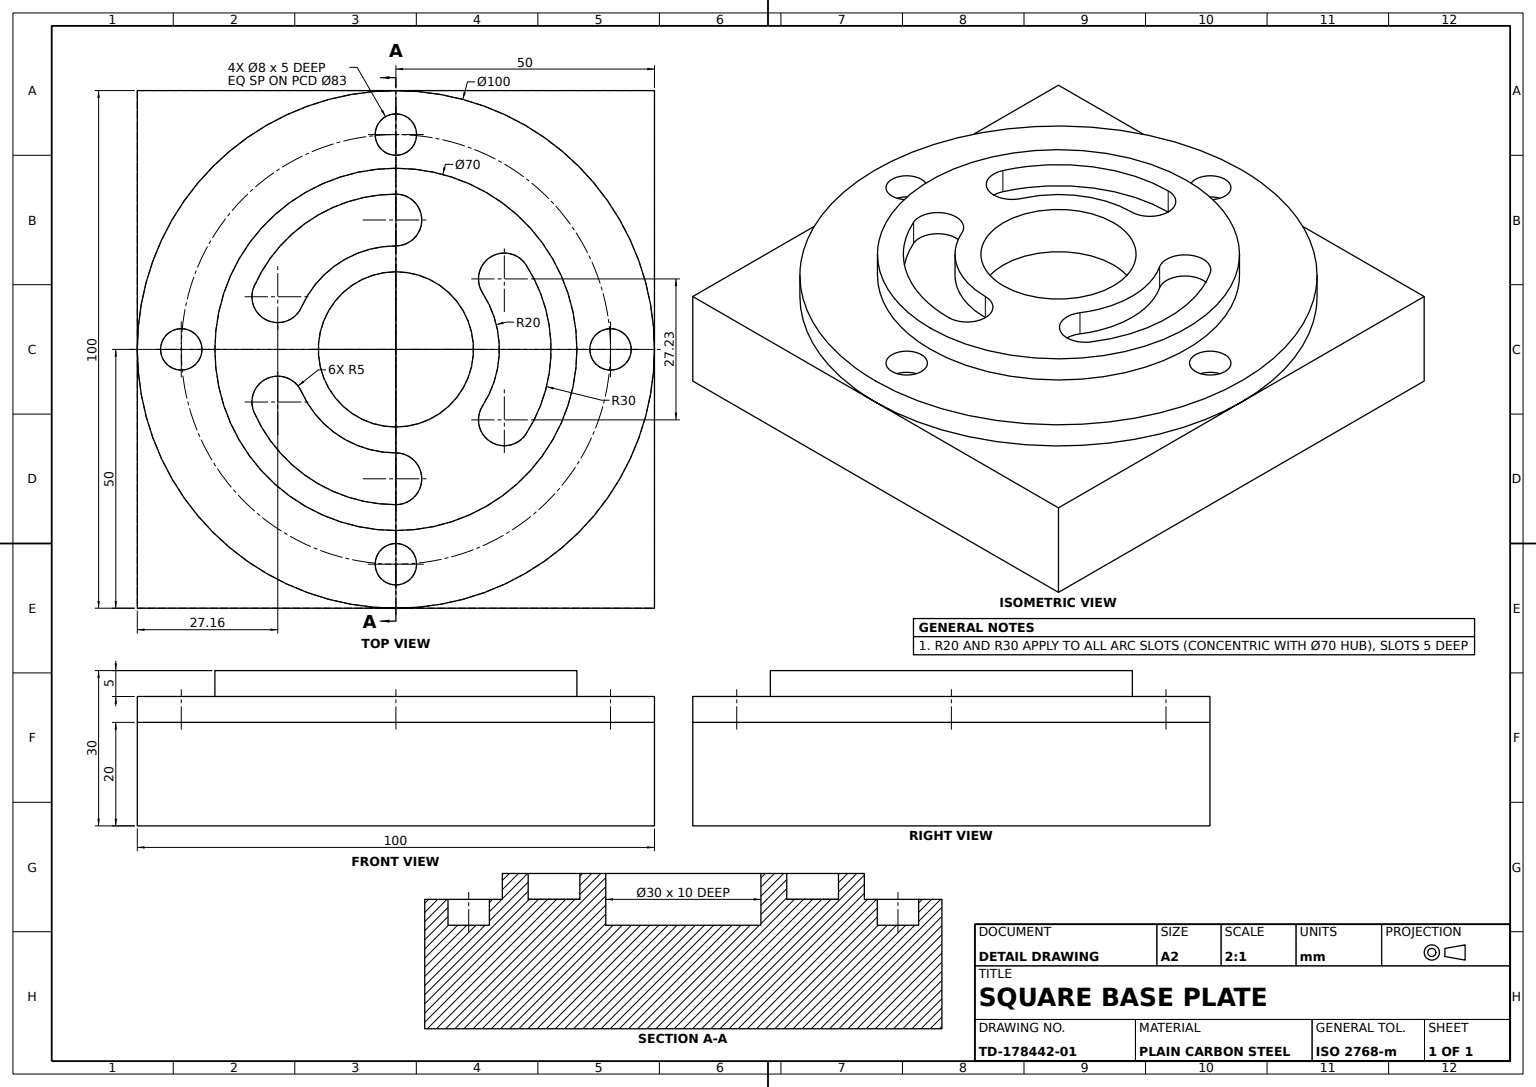
SolidWorks part; units mm, degrees
material "Plain Carbon Steel"
ref_plane "Front Plane" through (0, 0, 0) normal (0, 0, 1) x (1, 0, 0)
ref_plane "Top Plane" through (0, 0, 0) normal (0, 1, 0) x (1, 0, 0)
ref_plane "Right Plane" through (0, 0, 0) normal (1, 0, 0) x (0, 0, -1)
sketch "Base Plate Sketch" plane through (0, 0, 0) normal (0, 1, 0) x (1, 0, 0)
  line L1 (-50, 50) -> (50, 50)
  line L2 (-50, 50) -> (-50, -50)
  line L3 (-50, -50) -> (50, -50)
  line L4 (50, 50) -> (50, -50)
  line L5 (-50, 50) -> (50, -50) construction
  line L6 (-50, -50) -> (50, 50) construction
  point P0 (0, 0)
  dimension "D1" = 50
extrude "Base Plate" add sketch "Base Plate Sketch" along normal blind 20
sketch "Flange Disc Sketch" plane through (0, 20, 0) normal (0, 1, 0) x (1, 0, 0)
  circle A0 centre (0, 0) radius 50
  dimension "D1" = 100
extrude "Flange Disc" add sketch "Flange Disc Sketch" along normal blind 5
sketch "Flange Holes Sketch" plane through (0, 25, 0) normal (0, 1, 0) x (1, 0, 0)
  circle A0 centre (0, 0) radius 41.5 construction
  circle A1 centre (0, 41.5) radius 4
  circle A2 centre (41.5, 0) radius 4
  circle A3 centre (0, -41.5) radius 4
  circle A4 centre (-41.5, 0) radius 4
  dimension "D1" = 83
  dimension "D2" = 8
extrude "Flange Holes 4xØ8" cut sketch "Flange Holes Sketch" against normal blind 5
sketch "Hub Disc Sketch" plane through (0, 25, 0) normal (0, 1, 0) x (1, 0, 0)
  circle A0 centre (0, 0) radius 35
  dimension "D1" = 70
extrude "Hub Disc" add sketch "Hub Disc Sketch" along normal blind 5
sketch "Arc Slots Sketch" plane through (0, 30, 0) normal (0, 1, 0) x (1, 0, 0)
  line L3 (0, 30) -> (0, -35) construction
  circle A0 centre (0, 0) radius 25 construction
  arc A3 (-27.4052, -12.2047) -> (0, -30) centre (0, 0) ccw
  arc A4 (-18.2702, -8.1364) -> (0, -20) centre (0, 0) ccw
  arc A5 (16.7734, 10.8928) -> (25.1601, 16.3392) centre (20.9668, 13.616) cw
  arc A6 (16.7734, -10.8928) -> (25.1601, -16.3392) centre (20.9668, -13.616) ccw
  circle A7 centre (0, 0) radius 35 construction
  arc A8 (0, -20) -> (0, -30) centre (0, -25) cw
  arc A9 (-18.2702, -8.1364) -> (-27.4052, -12.2047) centre (-22.8377, -10.1705) ccw
  arc A10 (0, 30) -> (0, 20) centre (0, 25) cw
  arc A11 (-18.2702, 8.1364) -> (-27.4052, 12.2047) centre (-22.8377, 10.1705) cw
  arc A12 (0, 30) -> (-27.4052, 12.2047) centre (0, 0) ccw
  circle A13 centre (0, 0) radius 30 construction
  arc A14 (25.1601, -16.3392) -> (25.1601, 16.3392) centre (0, 0) ccw
  arc A15 (0, 20) -> (-18.2702, 8.1364) centre (0, 0) ccw
  circle A16 centre (0, 0) radius 20 construction
  arc A17 (16.7734, -10.8928) -> (16.7734, 10.8928) centre (0, 0) ccw
  point P6 (20, 0)
  point P37 (30, 0)
  dimension "D1" = 27.232
  dimension "D3" = 5
  dimension "D4" = 5
  dimension "D2" = 5
  dimension "D6" = 5
  dimension "D7" = 5
  dimension "D9" = 50
  dimension "D10" = 30
  dimension "D5" = 27.23
  dimension "D8" = 27.23
extrude "Arc Slots 3x" cut sketch "Arc Slots Sketch" against normal blind 5
sketch "Centre Bore Sketch" plane through (0, 30, 0) normal (0, 1, 0) x (1, 0, 0)
  circle A0 centre (0, 0) radius 15
  dimension "D1" = 30
extrude "Centre Bore" cut sketch "Centre Bore Sketch" against normal blind 10
